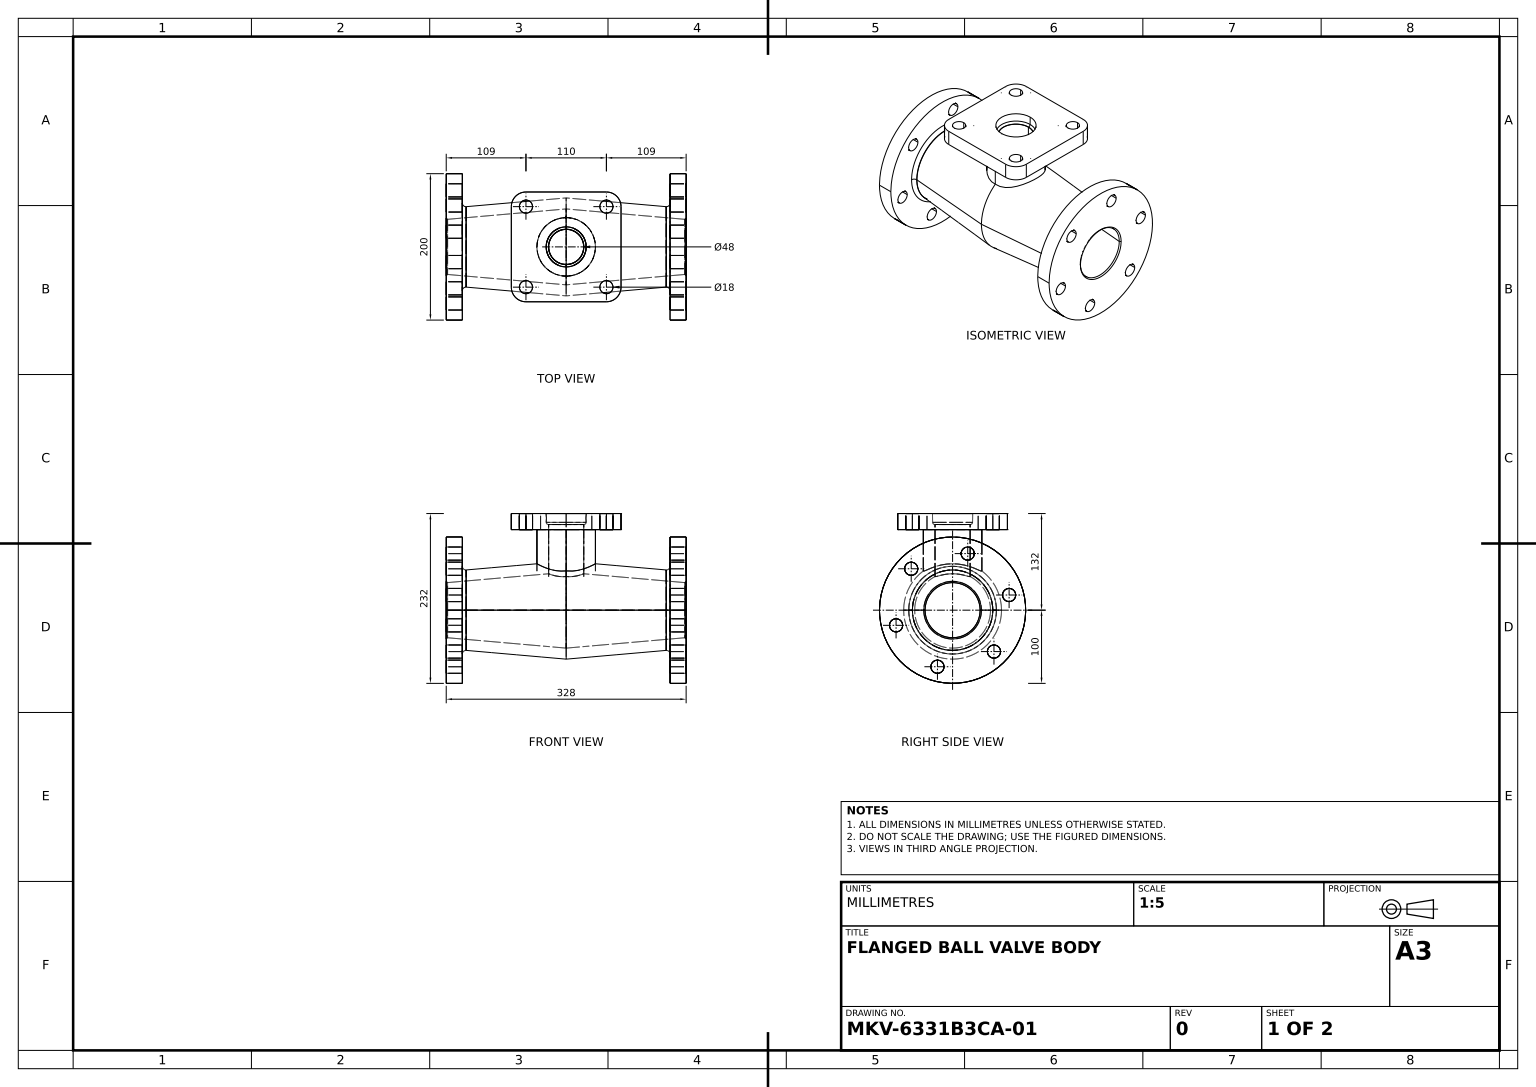
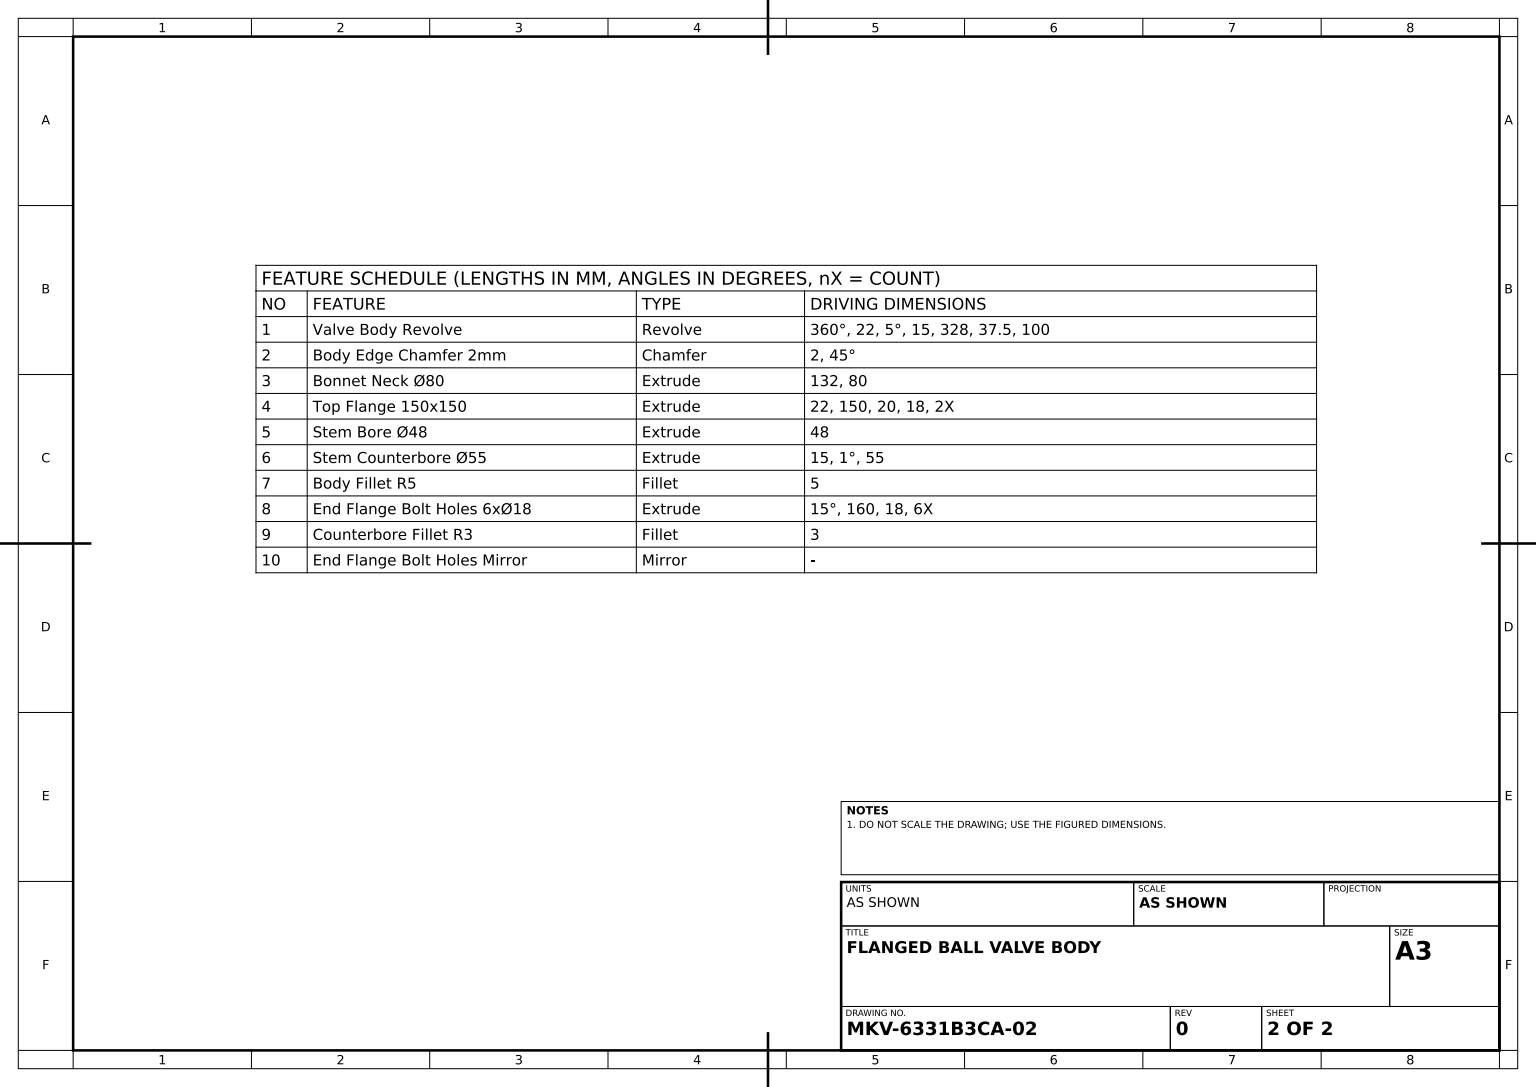
from build123d import *
from OCP.BRepFilletAPI import BRepFilletAPI_MakeChamfer

# Parameters (mm, degrees)
BODY_EDGE_CHAMFER_2MM_SIZE        = 2
BODY_EDGE_CHAMFER_2MM_SIZE2       = 1.846124693
BONNET_NECK_80_REACH              = 303.198
BONNET_NECK_SKETCH_R              = 40
TOP_FLANGE_SKETCH_R               = 9
TOP_FLANGE_150X150_DEPTH          = 22
STEM_BORE_48_REACH                = 303.198
STEM_BORE_SKETCH_R                = 24
STEM_COUNTERBORE_SKETCH_R         = 27.5
STEM_COUNTERBORE_55_DEPTH         = 15
STEM_COUNTERBORE_55_DRAFT         = -1
BODY_FILLET_R5_R                  = 5
END_FLANGE_BOLT_HOLES_6X_18_REACH = 369.434
END_FLANGE_BOLT_HOLES_SKETCH_R    = 9
COUNTERBORE_FILLET_R3_R           = 3


with BuildPart() as part:
    # Body Profile Sketch → Valve Body Revolve (revolve)
    with BuildSketch(Plane.XY, mode=Mode.PRIVATE) as valve_body_revolve_sk:
        Polygon((-142, -54.482048161), (0, -66.905438381), (142, -54.482048161), (142, -100), (164, -100), (164, -37.5), (0, -51.848140818), (-164, -37.5), (-164, -100), (-142, -100), align=None)
    revolve(valve_body_revolve_sk.sketch.rotate(Axis((-175.476190476, 0, 0), (1, 0, 0)), 270), axis=Axis((-175.476190476, 0, 0), (1, 0, 0)))

    # Body Edge Chamfer 2mm: one chamfer whose edges measure the first distance from different faces: ONE call of the kernel's chamfer builder (chamfer() names one face for all edges)
    body_edge_chamfer_2mm_edges_1 = [part.edges().sort_by_distance(p)[0] for p in [
        (164, 0, -37.5),
    ]]
    body_edge_chamfer_2mm_side_1 = [part.faces().sort_by_distance(p)[0] for p in [
        (82, 0, -44.674070409),
    ]]
    body_edge_chamfer_2mm_edges_2 = [part.edges().sort_by_distance(p)[0] for p in [
        (-164, 0, -37.5),
    ]]
    body_edge_chamfer_2mm_side_2 = [part.faces().sort_by_distance(p)[0] for p in [
        (-164, 0, -40.328427125),
    ]]
    body_edge_chamfer_2mm = BRepFilletAPI_MakeChamfer(part.part.solid().wrapped)
    for e in body_edge_chamfer_2mm_edges_1:
        body_edge_chamfer_2mm.Add(BODY_EDGE_CHAMFER_2MM_SIZE, BODY_EDGE_CHAMFER_2MM_SIZE2, e.wrapped, body_edge_chamfer_2mm_side_1[0].wrapped)  # the first distance lies on this face
    for e in body_edge_chamfer_2mm_edges_2:
        body_edge_chamfer_2mm.Add(BODY_EDGE_CHAMFER_2MM_SIZE, BODY_EDGE_CHAMFER_2MM_SIZE2, e.wrapped, body_edge_chamfer_2mm_side_2[0].wrapped)  # the first distance lies on this face
    add(Compound.cast(body_edge_chamfer_2mm.Shape()), mode=Mode.REPLACE)

    # Bonnet Neck Sketch → Bonnet Neck Ø80 (add, up to next)
    with BuildSketch(Plane(origin=(0, 132, 0), x_dir=(1, 0, 0), z_dir=(0, 1, 0)), mode=Mode.PRIVATE) as bonnet_neck_80_sk1:
        with Locations(Location((0, 0, 0), (0, 0, 270))):
            Circle(BONNET_NECK_SKETCH_R)
    bonnet_neck_80_tool1 = extrude(bonnet_neck_80_sk1.sketch, amount=-BONNET_NECK_80_REACH, mode=Mode.PRIVATE) - part.part
    add(bonnet_neck_80_tool1.solids().sort_by_distance((0, 132, 0))[0])

    # Top Flange Sketch → Top Flange 150x150 (add)
    with BuildSketch(Plane(origin=(0, 132, 0), x_dir=(1, 0, 0), z_dir=(0, 1, 0))):
        with BuildLine():
            Line((-55, -75), (55, -75))
            ThreePointArc((55, -75), (69.142135624, -69.142135624), (75, -55))
            Line((75, -55), (75, 55))
            ThreePointArc((75, 55), (69.142135624, 69.142135624), (55, 75))
            Line((55, 75), (-55, 75))
            ThreePointArc((-55, 75), (-69.142135624, 69.142135624), (-75, 55))
            Line((-75, 55), (-75, -55))
            ThreePointArc((-75, -55), (-69.142135624, -69.142135624), (-55, -75))
        make_face()
        with Locations(Location((-55, 55, 0), (0, 0, 270))):
            Circle(TOP_FLANGE_SKETCH_R, mode=Mode.SUBTRACT)
        with Locations(Location((55, 55, 0), (0, 0, 270))):
            Circle(TOP_FLANGE_SKETCH_R, mode=Mode.SUBTRACT)
        with Locations(Location((55, -55, 0), (0, 0, 270))):
            Circle(TOP_FLANGE_SKETCH_R, mode=Mode.SUBTRACT)
        with Locations(Location((-55, -55, 0), (0, 0, 270))):
            Circle(TOP_FLANGE_SKETCH_R, mode=Mode.SUBTRACT)
    extrude(amount=-TOP_FLANGE_150X150_DEPTH)

    # Stem Bore Sketch → Stem Bore Ø48 (cut, up to next)
    with BuildSketch(Plane(origin=(0, 132, 0), x_dir=(1, 0, 0), z_dir=(0, 1, 0)), mode=Mode.PRIVATE) as stem_bore_48_sk1:
        with Locations(Location((0, 0, 0), (0, 0, 270))):
            Circle(STEM_BORE_SKETCH_R)
    stem_bore_48_tool1 = extrude(stem_bore_48_sk1.sketch, amount=-STEM_BORE_48_REACH, mode=Mode.PRIVATE) & part.part
    add(stem_bore_48_tool1.solids().sort_by_distance((0, 132, 0))[0], mode=Mode.SUBTRACT)


with BuildPart() as stem_counterbore_55_tool:
    # Stem Counterbore Sketch → Stem Counterbore Ø55 (with draft: the straight prism first)
    with BuildSketch(Plane(origin=(0, 132, 0), x_dir=(1, 0, 0), z_dir=(0, 1, 0))):
        Circle(STEM_COUNTERBORE_SKETCH_R)
    extrude(amount=-STEM_COUNTERBORE_55_DEPTH)
    # Stem Counterbore Ø55: the draft: its side faces are tilted about the plane it starts from
    stem_counterbore_55_sides = [stem_counterbore_55_tool.faces().sort_by_distance(p)[0] for p in [
        (-27.5, 124.5, 0),
    ]]
    draft(stem_counterbore_55_sides, Plane(origin=(0, 132, 0), x_dir=(1, 0, 0), z_dir=(0, 1, 0)), STEM_COUNTERBORE_55_DRAFT)


with BuildPart() as part_1:
    add(part.part)

    # Stem Counterbore Ø55: cut by stem_counterbore_55_tool
    add(stem_counterbore_55_tool.part, mode=Mode.SUBTRACT)

    # Body Fillet R5
    body_fillet_r5_edges = [part_1.edges().sort_by_distance(p)[0] for p in [
        (-142, 0, -54.482048161),
        (142, 0, -54.482048161),
    ]]
    fillet(body_fillet_r5_edges, radius=BODY_FILLET_R5_R)

    # End Flange Bolt Holes Sketch → End Flange Bolt Holes 6xØ18 (cut, up to next)
    with BuildSketch(Plane(origin=(164, 0, 0), x_dir=(0, 0, -1), z_dir=(1, 0, 0)), mode=Mode.PRIVATE) as end_flange_bolt_holes_6x_18_sk1:
        with Locations((-77.274066103, -20.705523608)):
            Circle(END_FLANGE_BOLT_HOLES_SKETCH_R)
    end_flange_bolt_holes_6x_18_tool1 = extrude(end_flange_bolt_holes_6x_18_sk1.sketch, amount=-END_FLANGE_BOLT_HOLES_6X_18_REACH, mode=Mode.PRIVATE) & part_1.part
    # End Flange Bolt Holes Sketch → End Flange Bolt Holes 6xØ18 (cut, up to next)
    with BuildSketch(Plane(origin=(164, 0, 0), x_dir=(0, 0, -1), z_dir=(1, 0, 0)), mode=Mode.PRIVATE) as end_flange_bolt_holes_6x_18_sk2:
        with Locations((-56.568542495, 56.568542495)):
            Circle(END_FLANGE_BOLT_HOLES_SKETCH_R)
    end_flange_bolt_holes_6x_18_tool2 = extrude(end_flange_bolt_holes_6x_18_sk2.sketch, amount=-END_FLANGE_BOLT_HOLES_6X_18_REACH, mode=Mode.PRIVATE) & part_1.part
    # End Flange Bolt Holes Sketch → End Flange Bolt Holes 6xØ18 (cut, up to next)
    with BuildSketch(Plane(origin=(164, 0, 0), x_dir=(0, 0, -1), z_dir=(1, 0, 0)), mode=Mode.PRIVATE) as end_flange_bolt_holes_6x_18_sk3:
        with Locations((20.705523608, 77.274066103)):
            Circle(END_FLANGE_BOLT_HOLES_SKETCH_R)
    end_flange_bolt_holes_6x_18_tool3 = extrude(end_flange_bolt_holes_6x_18_sk3.sketch, amount=-END_FLANGE_BOLT_HOLES_6X_18_REACH, mode=Mode.PRIVATE) & part_1.part
    # End Flange Bolt Holes Sketch → End Flange Bolt Holes 6xØ18 (cut, up to next)
    with BuildSketch(Plane(origin=(164, 0, 0), x_dir=(0, 0, -1), z_dir=(1, 0, 0)), mode=Mode.PRIVATE) as end_flange_bolt_holes_6x_18_sk4:
        with Locations((77.274066103, 20.705523608)):
            Circle(END_FLANGE_BOLT_HOLES_SKETCH_R)
    end_flange_bolt_holes_6x_18_tool4 = extrude(end_flange_bolt_holes_6x_18_sk4.sketch, amount=-END_FLANGE_BOLT_HOLES_6X_18_REACH, mode=Mode.PRIVATE) & part_1.part
    # End Flange Bolt Holes Sketch → End Flange Bolt Holes 6xØ18 (cut, up to next)
    with BuildSketch(Plane(origin=(164, 0, 0), x_dir=(0, 0, -1), z_dir=(1, 0, 0)), mode=Mode.PRIVATE) as end_flange_bolt_holes_6x_18_sk5:
        with Locations((56.568542495, -56.568542495)):
            Circle(END_FLANGE_BOLT_HOLES_SKETCH_R)
    end_flange_bolt_holes_6x_18_tool5 = extrude(end_flange_bolt_holes_6x_18_sk5.sketch, amount=-END_FLANGE_BOLT_HOLES_6X_18_REACH, mode=Mode.PRIVATE) & part_1.part
    # End Flange Bolt Holes Sketch → End Flange Bolt Holes 6xØ18 (cut, up to next)
    with BuildSketch(Plane(origin=(164, 0, 0), x_dir=(0, 0, -1), z_dir=(1, 0, 0)), mode=Mode.PRIVATE) as end_flange_bolt_holes_6x_18_sk6:
        with Locations((-20.705523608, -77.274066103)):
            Circle(END_FLANGE_BOLT_HOLES_SKETCH_R)
    end_flange_bolt_holes_6x_18_tool6 = extrude(end_flange_bolt_holes_6x_18_sk6.sketch, amount=-END_FLANGE_BOLT_HOLES_6X_18_REACH, mode=Mode.PRIVATE) & part_1.part
    end_flange_bolt_holes_6x_18_1 = end_flange_bolt_holes_6x_18_tool1.solids().sort_by_distance((164, -20.705524, 77.274066))[0]
    add(end_flange_bolt_holes_6x_18_1, mode=Mode.SUBTRACT)
    end_flange_bolt_holes_6x_18_2 = end_flange_bolt_holes_6x_18_tool2.solids().sort_by_distance((164, 56.568542, 56.568542))[0]
    add(end_flange_bolt_holes_6x_18_2, mode=Mode.SUBTRACT)
    end_flange_bolt_holes_6x_18_3 = end_flange_bolt_holes_6x_18_tool3.solids().sort_by_distance((164, 77.274066, -20.705524))[0]
    add(end_flange_bolt_holes_6x_18_3, mode=Mode.SUBTRACT)
    end_flange_bolt_holes_6x_18_4 = end_flange_bolt_holes_6x_18_tool4.solids().sort_by_distance((164, 20.705524, -77.274066))[0]
    add(end_flange_bolt_holes_6x_18_4, mode=Mode.SUBTRACT)
    end_flange_bolt_holes_6x_18_5 = end_flange_bolt_holes_6x_18_tool5.solids().sort_by_distance((164, -56.568542, -56.568542))[0]
    add(end_flange_bolt_holes_6x_18_5, mode=Mode.SUBTRACT)
    end_flange_bolt_holes_6x_18_6 = end_flange_bolt_holes_6x_18_tool6.solids().sort_by_distance((164, -77.274066, 20.705524))[0]
    add(end_flange_bolt_holes_6x_18_6, mode=Mode.SUBTRACT)
    end_flange_bolt_holes_6x_18 = end_flange_bolt_holes_6x_18_1 + end_flange_bolt_holes_6x_18_2 + end_flange_bolt_holes_6x_18_3 + end_flange_bolt_holes_6x_18_4 + end_flange_bolt_holes_6x_18_5 + end_flange_bolt_holes_6x_18_6  # End Flange Bolt Holes 6xØ18 as one shape, for the pattern or mirror that repeats it

    # Counterbore Fillet R3
    counterbore_fillet_r3_edges = [part_1.edges().sort_by_distance(p)[0] for p in [
        (-27.238174026, 117, 0),
    ]]
    fillet(counterbore_fillet_r3_edges, radius=COUNTERBORE_FILLET_R3_R)

    # End Flange Bolt Holes Mirror: End Flange Bolt Holes 6xØ18 across plane
    add(end_flange_bolt_holes_6x_18.mirror(Plane(origin=(0, 0, 0), x_dir=(0, 0, 1), z_dir=(1, 0, 0))), mode=Mode.SUBTRACT)


solid = part_1.part
